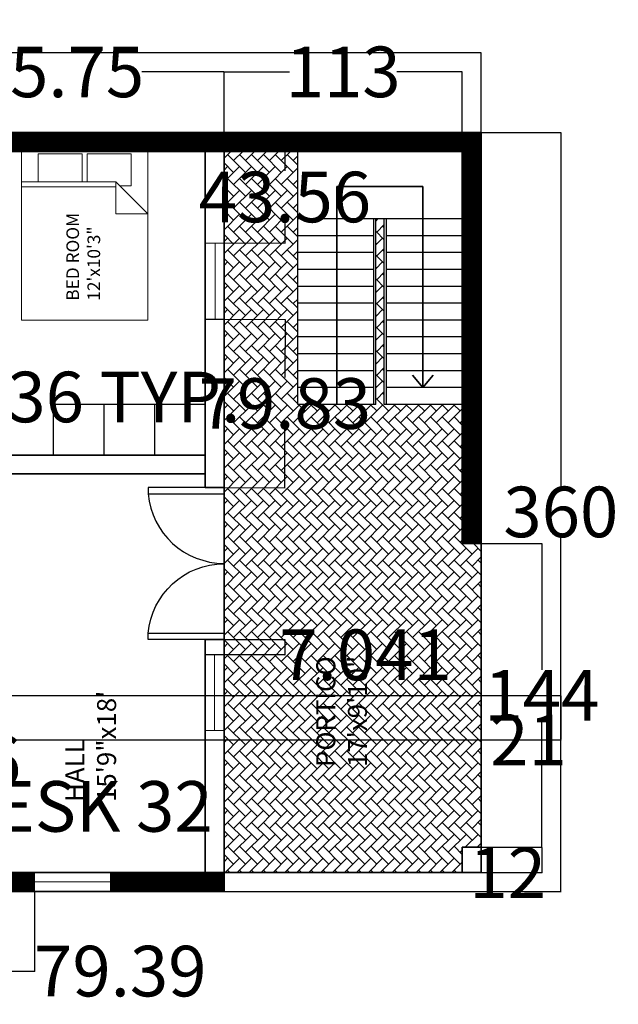
# Model space of a CAD drawing. Units: inches. Extents: x -1226 to 4538, y -998 to 1029.
# Tile 4 of 5: x -658 to -374, y -998 to -531. Entities that reach past the tile are written whole.
import ezdxf

# ---------------------------------------------------------------- set-up
doc = ezdxf.new("R2010")
doc.units = ezdxf.units.IN
doc.header["$MEASUREMENT"] = 0
for name, color, linetype, lineweight in [('A-ANNO-DIMS', 2, 'Continuous', 18), ('A-ANNO-SYMB', 7, 'Continuous', 35), ('A-AREA-IDEN', 7, 'Continuous', 18), ('A-DOOR', 4, 'Continuous', 25), ('A-FLOR-CASE', 8, 'Continuous', 25), ('A-FLOR-PATT', 2, 'Continuous', 13), ('A-FLOR-STRS', 7, 'Continuous', 25), ('A-FURN', 8, 'Continuous', 18), ('A-GLAZ', 3, 'Continuous', 18), ('A-WALL', 7, 'Continuous', 35), ('A-WALL-PATT', 1, 'Continuous', 13)]:
    doc.layers.add(name, color=color, linetype=linetype, lineweight=lineweight)
doc.styles.get("Standard").update_dxf_attribs({"font": 'arial.ttf'})
doc.dimstyles.get("Standard").update_dxf_attribs({"dimtxt": 24, "dimasz": 0.18, "dimexe": 0.18, "dimexo": 0.0625, "dimgap": 0.09, "dimtad": 0, "dimtih": 1, "dimtoh": 1, "dimdec": 0, "dimzin": 0, "dimdsep": 46, "dimlunit": 4, "dimtxsty": 'Standard', "dimcen": 0.09, "dimadec": 0, "dimazin": 0, "dimtfac": 1, "dimtdec": 0, "dimtofl": 0, "dimtmove": 0, "dimatfit": 3, "dimfxl": 1, "dimtolj": 1, "dimtzin": 0, "dimarcsym": 0})

# ---------------------------------------------------------------- blocks, each defined once
blk = doc.blocks.new('Bed - Queen')
for p, q in [((0, -80.00003), (0, 0)), ((0, 0), (59.99999, 0)), ((59.99999, 0), (59.99999, -80.00003)), ((7.99999, -1.2), (28.79998, -1.2)), ((7.99999, -14.4), (7.99999, -1.2)), ((28.79998, -1.2), (28.79998, -14.4)), ((31.19999, -1.2), (51.99999, -1.2)), ((31.19999, -14.4), (31.19999, -1.2)), ((51.99999, -1.2), (51.99999, -16.4)), ((0, -14.4), (44.8, -14.4)), ((44.8, -16.8), (0, -16.8)), ((59.99999, -29.6), (44.8, -14.4)), ((44.8, -14.4), (44.8, -29.6)), ((51.99999, -16.4), (46.79936, -16.4)), ((44.8, -29.6), (59.99999, -29.6)), ((59.99999, -80.00003), (0, -80.00003))]:
    blk.add_line(p, q)
blk = doc.blocks.new('DOOR-SWING-36')
for p, q in [((36, 36), (0, 36)), ((0, 36), (0, 33)), ((0, 33), (36, 33)), ((36, 33), (36, 36))]:
    blk.add_line(p, q)
blk.add_arc((36, 36.14), 36.14, 184.9791, 270)
blk = doc.blocks.new('WIN-36')
for p, q in [((0, 36), (9, 36)), ((4.5, 0), (4.5, 36)), ((0, 0), (9, 0))]:
    blk.add_line(p, q)
blk = doc.blocks.new('WARDROBE-72X24')
for p, q in [((72, 24), (0, 24)), ((0, 24), (0, 0)), ((24, 24), (24, 0)), ((48, 24), (48, 0)), ((72, 0), (72, 24)), ((0, 0), (72, 0))]:
    blk.add_line(p, q)
blk = doc.blocks.new('STAIR-RETURN-120X78')
for p, q in [((0, 0), (0, 120)), ((0, 120), (78, 120)), ((78, 120), (78, 0)), ((42, 88), (0, 88)), ((36, 0), (36, 88)), ((37, 0), (37, 88)), ((41, 0), (41, 88)), ((42, 0), (42, 88)), ((78, 88), (42, 88)), ((36, 80), (0, 80)), ((78, 80), (42, 80)), ((36, 72), (0, 72)), ((78, 72), (42, 72)), ((36, 64), (0, 64)), ((78, 64), (42, 64)), ((36, 56), (0, 56)), ((78, 56), (42, 56)), ((36, 48), (0, 48)), ((78, 48), (42, 48)), ((36, 40), (0, 40)), ((78, 40), (42, 40)), ((36, 32), (0, 32)), ((78, 32), (42, 32)), ((36, 24), (0, 24)), ((78, 24), (42, 24)), ((36, 16), (0, 16)), ((78, 16), (42, 16)), ((36, 8), (0, 8)), ((78, 8), (42, 8)), ((37, 0), (0, 0)), ((78, 0), (41, 0))]:
    blk.add_line(p, q)
blk = doc.blocks.new('STAIR-DIRECTION-RETURN')
for p, q in [((0, 0), (0, 103.3)), ((0, 103.3), (40.82, 103.3)), ((40.82, 103.3), (40.82, 8)), ((40.82, 8), (35.91, 13.94)), ((40.82, 8), (45.74, 13.94))]:
    blk.add_line(p, q)
blk = doc.blocks.new('*D26')
at = {"layer": 'A-ANNO-DIMS', "color": 0, "lineweight": -2, "transparency": 16777216}
for p, q in [((-694.2, -692), (-699.72, -692)), ((-699.54, -692.18), (-699.54, -697.48)), ((-699.54, -727.82), (-699.54, -722.51)), ((-694.2, -728), (-699.72, -728))]:
    blk.add_line(p, q, dxfattribs=at)
at = {"layer": 'A-ANNO-DIMS', "color": 0, "transparency": 16777216}
for points in [[(-699.57, -692.18), (-699.51, -692.18), (-699.54, -692)], [(-699.57, -727.82), (-699.51, -727.82), (-699.54, -728)]]:
    blk.add_solid(points, dxfattribs=at)
at = {"layer": 'Defpoints', "color": 0, "transparency": 16777216}
for p in [(-694.14, -692), (-699.54, -728), (-694.14, -728)]:
    blk.add_point(p, dxfattribs=at)
at = {"layer": 'A-ANNO-DIMS', "color": 0, "transparency": 16777216, "insert": (-699.54, -710), "char_height": 24, "attachment_point": 5}
blk.add_mtext('\\A1;DOOR LEAF 36 TYP.', dxfattribs=at)
blk = doc.blocks.new('*D44')
at = {"layer": 'A-ANNO-DIMS', "color": 0, "lineweight": -2, "transparency": 16777216}
for p, q in [((-728.59, -899.5), (-728.59, -904.39)), ((-696.71, -899.5), (-696.71, -904.39)), ((-728.41, -904.21), (-696.89, -904.21)), ((-696.71, -904.21), (-696.53, -904.21))]:
    blk.add_line(p, q, dxfattribs=at)
at = {"layer": 'A-ANNO-DIMS', "color": 0, "transparency": 16777216}
for points in [[(-728.41, -904.18), (-728.41, -904.24), (-728.59, -904.21)], [(-696.89, -904.18), (-696.89, -904.24), (-696.71, -904.21)]]:
    blk.add_solid(points, dxfattribs=at)
at = {"layer": 'Defpoints', "color": 0, "transparency": 16777216}
for p in [(-728.59, -899.43), (-696.71, -899.43), (-696.71, -904.21)]:
    blk.add_point(p, dxfattribs=at)
at = {"layer": 'A-ANNO-DIMS', "color": 0, "transparency": 16777216, "insert": (-629.67, -904.21), "char_height": 24, "attachment_point": 5}
blk.add_mtext('\\A1;DESK 32', dxfattribs=at)
blk = doc.blocks.new('*D45')
at = {"layer": 'A-ANNO-DIMS', "color": 0, "lineweight": -2, "transparency": 16777216}
for p, q in [((-696.65, -882.96), (-691.75, -882.96)), ((-691.93, -882.96), (-691.93, -882.78)), ((-691.93, -882.78), (-691.75, -882.78)), ((-691.93, -899.25), (-691.93, -883.14)), ((-696.65, -899.43), (-691.75, -899.43))]:
    blk.add_line(p, q, dxfattribs=at)
at = {"layer": 'A-ANNO-DIMS', "color": 0, "transparency": 16777216}
for points in [[(-691.96, -883.14), (-691.9, -883.14), (-691.93, -882.96)], [(-691.96, -899.25), (-691.9, -899.25), (-691.93, -899.43)]]:
    blk.add_solid(points, dxfattribs=at)
at = {"layer": 'Defpoints', "color": 0, "transparency": 16777216}
for p in [(-696.71, -882.96), (-691.93, -882.96), (-696.71, -899.43)]:
    blk.add_point(p, dxfattribs=at)
at = {"layer": 'A-ANNO-DIMS', "color": 0, "transparency": 16777216, "insert": (-675.61, -882.78), "char_height": 24, "attachment_point": 5}
blk.add_mtext('\\A1;16', dxfattribs=at)
blk = doc.blocks.new('*D48')
at = {"layer": 'A-ANNO-DIMS', "color": 0, "lineweight": -2, "transparency": 16777216}
for p, q in [((-1061.17, -584.46), (-1061.17, -546.6)), ((-1060.99, -546.78), (-776.71, -546.78)), ((-439.35, -546.78), (-723.62, -546.78)), ((-439.17, -584.46), (-439.17, -546.6))]:
    blk.add_line(p, q, dxfattribs=at)
at = {"layer": 'A-ANNO-DIMS', "color": 0, "transparency": 16777216}
for points in [[(-1060.99, -546.75), (-1060.99, -546.81), (-1061.17, -546.78)], [(-439.35, -546.75), (-439.35, -546.81), (-439.17, -546.78)]]:
    blk.add_solid(points, dxfattribs=at)
at = {"layer": 'Defpoints', "color": 0, "transparency": 16777216}
for p in [(-439.17, -546.78), (-1061.17, -584.53), (-439.17, -584.53)]:
    blk.add_point(p, dxfattribs=at)
at = {"layer": 'A-ANNO-DIMS', "color": 0, "transparency": 16777216, "insert": (-750.17, -546.78), "char_height": 24, "attachment_point": 5}
blk.add_mtext('\\A1;622', dxfattribs=at)
blk = doc.blocks.new('*D49')
at = {"layer": 'A-ANNO-DIMS', "color": 0, "lineweight": -2, "transparency": 16777216}
for p, q in [((-439.1, -584.53), (-401.24, -584.53)), ((-401.42, -584.71), (-401.42, -752.18)), ((-401.42, -944.35), (-401.42, -776.88)), ((-561.1, -944.53), (-401.24, -944.53))]:
    blk.add_line(p, q, dxfattribs=at)
at = {"layer": 'A-ANNO-DIMS', "color": 0, "transparency": 16777216}
for points in [[(-401.45, -584.71), (-401.39, -584.71), (-401.42, -584.53)], [(-401.45, -944.35), (-401.39, -944.35), (-401.42, -944.53)]]:
    blk.add_solid(points, dxfattribs=at)
at = {"layer": 'Defpoints', "color": 0, "transparency": 16777216}
for p in [(-439.17, -584.53), (-561.17, -944.53), (-401.42, -944.53)]:
    blk.add_point(p, dxfattribs=at)
at = {"layer": 'A-ANNO-DIMS', "color": 0, "transparency": 16777216, "insert": (-401.42, -764.53), "char_height": 24, "attachment_point": 5}
blk.add_mtext('\\A1;360', dxfattribs=at)
blk = doc.blocks.new('*D54')
at = {"layer": 'A-ANNO-DIMS', "color": 0, "lineweight": -2, "transparency": 16777216}
for p, q in [((-736.92, -593.48), (-736.92, -555.62)), ((-736.74, -555.8), (-697.91, -555.79)), ((-561.35, -555.78), (-600.18, -555.78)), ((-561.17, -593.46), (-561.17, -555.6))]:
    blk.add_line(p, q, dxfattribs=at)
at = {"layer": 'A-ANNO-DIMS', "color": 0, "transparency": 16777216}
for points in [[(-736.74, -555.77), (-736.74, -555.83), (-736.92, -555.8)], [(-561.35, -555.75), (-561.35, -555.81), (-561.17, -555.78)]]:
    blk.add_solid(points, dxfattribs=at)
at = {"layer": 'Defpoints', "color": 0, "transparency": 16777216}
for p in [(-561.17, -555.78), (-736.92, -593.55), (-561.17, -593.53)]:
    blk.add_point(p, dxfattribs=at)
at = {"layer": 'A-ANNO-DIMS', "color": 0, "transparency": 16777216, "insert": (-649.05, -555.79), "char_height": 24, "attachment_point": 5}
blk.add_mtext('\\A1;175.75', dxfattribs=at)
blk = doc.blocks.new('*D55')
at = {"layer": 'A-ANNO-DIMS', "color": 0, "lineweight": -2, "transparency": 16777216}
for p, q in [((-561.17, -593.46), (-561.17, -555.6)), ((-560.99, -555.78), (-530.14, -555.78)), ((-448.35, -555.78), (-479.19, -555.78)), ((-448.17, -593.46), (-448.17, -555.6))]:
    blk.add_line(p, q, dxfattribs=at)
at = {"layer": 'A-ANNO-DIMS', "color": 0, "transparency": 16777216}
for points in [[(-560.99, -555.75), (-560.99, -555.81), (-561.17, -555.78)], [(-448.35, -555.75), (-448.35, -555.81), (-448.17, -555.78)]]:
    blk.add_solid(points, dxfattribs=at)
at = {"layer": 'Defpoints', "color": 0, "transparency": 16777216}
for p in [(-448.17, -555.78), (-561.17, -593.53), (-448.17, -593.53)]:
    blk.add_point(p, dxfattribs=at)
at = {"layer": 'A-ANNO-DIMS', "color": 0, "transparency": 16777216, "insert": (-504.67, -555.78), "char_height": 24, "attachment_point": 5}
blk.add_mtext('\\A1;113', dxfattribs=at)
blk = doc.blocks.new('*D58')
at = {"layer": 'A-ANNO-DIMS', "color": 0, "lineweight": -2, "transparency": 16777216}
for p, q in [((-730.47, -944.64), (-730.47, -982.51)), ((-651.08, -944.55), (-651.08, -982.51)), ((-730.29, -982.33), (-651.26, -982.33)), ((-651.08, -982.33), (-650.9, -982.33))]:
    blk.add_line(p, q, dxfattribs=at)
at = {"layer": 'A-ANNO-DIMS', "color": 0, "transparency": 16777216}
for points in [[(-730.29, -982.3), (-730.29, -982.36), (-730.47, -982.33)], [(-651.26, -982.3), (-651.26, -982.36), (-651.08, -982.33)]]:
    blk.add_solid(points, dxfattribs=at)
at = {"layer": 'Defpoints', "color": 0, "transparency": 16777216}
for p in [(-730.47, -944.58), (-651.08, -944.48), (-651.08, -982.33)]:
    blk.add_point(p, dxfattribs=at)
at = {"layer": 'A-ANNO-DIMS', "color": 0, "transparency": 16777216, "insert": (-610.39, -982.33), "char_height": 24, "attachment_point": 5}
blk.add_mtext('\\A1;79.39', dxfattribs=at)
blk = doc.blocks.new('*D62')
at = {"layer": 'A-ANNO-DIMS', "color": 0, "lineweight": -2, "transparency": 16777216}
for p, q in [((-448.1, -779.53), (-410.24, -779.53)), ((-410.42, -779.71), (-410.42, -839.39)), ((-410.42, -923.35), (-410.42, -863.67)), ((-448.1, -923.53), (-410.24, -923.53))]:
    blk.add_line(p, q, dxfattribs=at)
at = {"layer": 'A-ANNO-DIMS', "color": 0, "transparency": 16777216}
for points in [[(-410.45, -779.71), (-410.39, -779.71), (-410.42, -779.53)], [(-410.45, -923.35), (-410.39, -923.35), (-410.42, -923.53)]]:
    blk.add_solid(points, dxfattribs=at)
at = {"layer": 'Defpoints', "color": 0, "transparency": 16777216}
for p in [(-448.17, -779.53), (-448.17, -923.53), (-410.42, -923.53)]:
    blk.add_point(p, dxfattribs=at)
at = {"layer": 'A-ANNO-DIMS', "color": 0, "transparency": 16777216, "insert": (-410.42, -851.53), "char_height": 24, "attachment_point": 5}
blk.add_mtext('\\A1;144', dxfattribs=at)
blk = doc.blocks.new('*D63')
at = {"layer": 'A-ANNO-DIMS', "color": 0, "lineweight": -2, "transparency": 16777216}
for p, q in [((-448.1, -923.53), (-410.24, -923.53)), ((-410.42, -923.71), (-410.42, -935.35)), ((-448.1, -935.53), (-410.24, -935.53)), ((-410.42, -935.71), (-410.6, -935.71)), ((-410.42, -935.53), (-410.42, -935.71))]:
    blk.add_line(p, q, dxfattribs=at)
at = {"layer": 'A-ANNO-DIMS', "color": 0, "transparency": 16777216}
for points in [[(-410.45, -923.71), (-410.39, -923.71), (-410.42, -923.53)], [(-410.45, -935.35), (-410.39, -935.35), (-410.42, -935.53)]]:
    blk.add_solid(points, dxfattribs=at)
at = {"layer": 'Defpoints', "color": 0, "transparency": 16777216}
for p in [(-448.17, -923.53), (-448.17, -935.53), (-410.42, -935.53)]:
    blk.add_point(p, dxfattribs=at)
at = {"layer": 'A-ANNO-DIMS', "color": 0, "transparency": 16777216, "insert": (-426.62, -935.71), "char_height": 24, "attachment_point": 5}
blk.add_mtext('\\A1;12', dxfattribs=at)
blk = doc.blocks.new('*D64')
at = {"layer": 'A-ANNO-DIMS', "color": 0, "lineweight": -2, "transparency": 16777216}
for p, q in [((-570.1, -593.53), (-532.24, -593.36)), ((-532.42, -593.54), (-532.37, -602.79)), ((-532.22, -636.74), (-532.26, -627.49)), ((-569.91, -637.09), (-532.04, -636.92))]:
    blk.add_line(p, q, dxfattribs=at)
at = {"layer": 'A-ANNO-DIMS', "color": 0, "transparency": 16777216}
for points in [[(-532.39, -593.54), (-532.45, -593.54), (-532.42, -593.36)], [(-532.19, -636.74), (-532.25, -636.74), (-532.22, -636.92)]]:
    blk.add_solid(points, dxfattribs=at)
at = {"layer": 'Defpoints', "color": 0, "transparency": 16777216}
for p in [(-570.17, -593.53), (-569.97, -637.09), (-532.22, -636.92)]:
    blk.add_point(p, dxfattribs=at)
at = {"layer": 'A-ANNO-DIMS', "color": 0, "transparency": 16777216, "insert": (-532.32, -615.14), "char_height": 24, "attachment_point": 5}
blk.add_mtext('\\A1;43.56', dxfattribs=at)
blk = doc.blocks.new('*D65')
at = {"layer": 'A-ANNO-DIMS', "color": 0, "lineweight": -2, "transparency": 16777216}
for p, q in [((-569.91, -673.09), (-532.04, -673.18)), ((-532.22, -673.36), (-532.29, -700.75)), ((-532.42, -752.84), (-532.35, -725.45)), ((-570.1, -752.93), (-532.24, -753.02))]:
    blk.add_line(p, q, dxfattribs=at)
at = {"layer": 'A-ANNO-DIMS', "color": 0, "transparency": 16777216}
for points in [[(-532.25, -673.36), (-532.19, -673.36), (-532.22, -673.18)], [(-532.45, -752.84), (-532.39, -752.84), (-532.42, -753.02)]]:
    blk.add_solid(points, dxfattribs=at)
at = {"layer": 'Defpoints', "color": 0, "transparency": 16777216}
for p in [(-569.97, -673.09), (-570.17, -752.93), (-532.42, -753.02)]:
    blk.add_point(p, dxfattribs=at)
at = {"layer": 'A-ANNO-DIMS', "color": 0, "transparency": 16777216, "insert": (-532.32, -713.1), "char_height": 24, "attachment_point": 5}
blk.add_mtext('\\A1;79.83', dxfattribs=at)
blk = doc.blocks.new('*D66')
at = {"layer": 'A-ANNO-DIMS', "color": 0, "lineweight": -2, "transparency": 16777216}
for p, q in [((-570.1, -825.1), (-532.24, -825.06)), ((-532.42, -825.24), (-532.41, -831.92)), ((-570.1, -832.14), (-532.23, -832.1)), ((-532.41, -832.1), (-532.41, -832.28)), ((-532.41, -832.28), (-532.23, -832.28))]:
    blk.add_line(p, q, dxfattribs=at)
at = {"layer": 'A-ANNO-DIMS', "color": 0, "transparency": 16777216}
for points in [[(-532.39, -825.24), (-532.45, -825.24), (-532.42, -825.06)], [(-532.38, -831.92), (-532.44, -831.92), (-532.41, -832.1)]]:
    blk.add_solid(points, dxfattribs=at)
at = {"layer": 'Defpoints', "color": 0, "transparency": 16777216}
for p in [(-570.17, -825.1), (-570.16, -832.14), (-532.41, -832.1)]:
    blk.add_point(p, dxfattribs=at)
at = {"layer": 'A-ANNO-DIMS', "color": 0, "transparency": 16777216, "insert": (-494.06, -832.28), "char_height": 24, "attachment_point": 5}
blk.add_mtext('\\A1;7.041', dxfattribs=at)
blk = doc.blocks.new('*D78')
at = {"layer": 'A-ANNO-DIMS', "color": 0, "lineweight": -2, "transparency": 16777216}
for p, q in [((-1028.09, -851.56), (-401.24, -851.56)), ((-401.42, -851.74), (-401.42, -872.38)), ((-1028.09, -872.56), (-401.24, -872.56)), ((-401.42, -872.74), (-401.6, -872.74)), ((-401.42, -872.56), (-401.42, -872.74))]:
    blk.add_line(p, q, dxfattribs=at)
at = {"layer": 'A-ANNO-DIMS', "color": 0, "transparency": 16777216}
for points in [[(-401.45, -851.74), (-401.39, -851.74), (-401.42, -851.56)], [(-401.45, -872.38), (-401.39, -872.38), (-401.42, -872.56)]]:
    blk.add_solid(points, dxfattribs=at)
at = {"layer": 'Defpoints', "color": 0, "transparency": 16777216}
for p in [(-1028.16, -851.56), (-1028.16, -872.56), (-401.42, -872.56)]:
    blk.add_point(p, dxfattribs=at)
at = {"layer": 'A-ANNO-DIMS', "color": 0, "transparency": 16777216, "insert": (-416.76, -872.74), "char_height": 24, "attachment_point": 5}
blk.add_mtext('\\A1;21', dxfattribs=at)

msp = doc.modelspace()

# ---------------------------------------------------------------- hatches: boundary and pattern name
at = {"layer": 'A-FLOR-PATT'}
h = msp.add_hatch(dxfattribs=at)
h.set_pattern_fill('AR-HBONE', color=256, angle=90)
h.set_pattern_definition([(135, (-1048.8063, 527.8678), (-5.656854, 3e-16), [12, -4]), (225, (-1051.6348, 530.696), (-5.656854, 8e-16), [12, -4])])
h.paths.add_polyline_path([(-526.1662, -713.5274), (-526.1662, -593.5274), (-561.1662, -593.5274), (-561.1662, -752.9256), (-561.1621, -752.9256), (-561.1621, -755.9256), (-561.1635, -822.1022), (-561.1621, -822.1022), (-561.1621, -825.1022), (-561.1658, -935.5274), (-448.1662, -935.5274), (-448.1662, -923.5274), (-439.1662, -923.5274), (-439.1662, -779.5274), (-448.1662, -779.5274), (-448.1662, -713.5274), (-485.1662, -713.5274), (-485.1662, -625.5274), (-489.1662, -625.5274), (-489.1662, -713.5274)])
h.paths.add_polyline_path([(-488.2978, -889.1778), (-488.2978, -827.0005), (-521.881, -827.0005), (-521.881, -889.1778)], flags=24)
at = {"layer": 'A-WALL-PATT'}
h = msp.add_hatch(dxfattribs=at)
h.set_pattern_fill('ANSI31', color=256, angle=90)
h.set_pattern_definition([(135, (-1048.80633, 527.86775), (-0.088388348, -0.088388348), [])])
h.paths.add_polyline_path([(-1052.1662, -935.5274), (-1052.1662, -878.4295), (-1061.1662, -878.4295), (-1061.1662, -944.5274), (-1012.2132, -944.5274), (-1012.2132, -935.5274)])
h.paths.add_polyline_path([(-976.2132, -935.5274), (-976.2132, -944.5274), (-730.4734, -944.5274), (-730.4734, -935.5274)])
h.paths.add_polyline_path([(-694.4734, -935.5274), (-694.4734, -944.5274), (-651.0832, -944.5274), (-651.0832, -935.5274)])
h.paths.add_polyline_path([(-615.0832, -935.5274), (-615.0832, -944.5274), (-561.1662, -944.5274), (-561.1662, -935.5274)])
h.paths.add_polyline_path([(-712.9165, -584.5274), (-712.9165, -593.5274), (-657.3138, -593.5274), (-657.3138, -593.4838), (-597.3139, -593.4838), (-448.1662, -593.5274), (-448.1662, -713.5274), (-448.1662, -779.5274), (-439.1662, -779.5274), (-439.1662, -584.5274)])
h.paths.add_polyline_path([(-875.9292, -584.5274), (-875.9292, -593.5274), (-736.9165, -593.5274), (-736.9165, -584.5274)])
h.paths.add_polyline_path([(-950.5052, -584.5274), (-950.5052, -593.5274), (-911.9292, -593.5274), (-911.9292, -584.5274)])
h.paths.add_polyline_path([(-1011.0429, -584.5274), (-1011.0429, -593.5274), (-974.5052, -593.5274), (-974.5052, -584.5274)])
h.paths.add_polyline_path([(-1061.1662, -584.5274), (-1061.1662, -693.4459), (-1052.1662, -693.4459), (-1052.1662, -593.5274), (-1035.0429, -593.5274), (-1035.0429, -584.5274)])
h.paths.add_polyline_path([(-1061.1662, -795.2404), (-1061.1662, -842.4295), (-1052.1662, -842.4295), (-1052.1662, -795.2404)])
h.paths.add_polyline_path([(-1061.1662, -717.4459), (-1061.1662, -739.4249), (-1052.1662, -739.4249), (-1052.1662, -717.4459)])

# ---------------------------------------------------------------- linework, layer by layer
at = {"layer": 'A-WALL'}
for p, q in [((-1061.1662, -584.5274), (-439.1662, -584.5274)), ((-439.1662, -935.5274), (-439.1662, -584.5274)), ((-1052.1662, -593.5274), (-448.1662, -593.5274)), ((-570.1662, -752.9256), (-570.1662, -593.5274)), ((-561.1662, -944.5274), (-561.1662, -593.5274)), ((-448.1662, -779.5274), (-448.1662, -593.5274)), ((-685.1662, -737.5274), (-570.1662, -737.5274)), ((-694.1662, -746.5274), (-570.1662, -746.5274)), ((-448.1662, -779.5274), (-439.1662, -779.5274)), ((-570.1662, -935.5274), (-570.1662, -825.1022)), ((-448.1662, -935.5274), (-448.1662, -923.5274)), ((-448.1662, -923.5274), (-439.1662, -923.5274)), ((-1052.1662, -935.5274), (-439.1662, -935.5274)), ((-1061.1662, -944.5274), (-561.1662, -944.5274))]:
    msp.add_line(p, q, dxfattribs=at)

# ---------------------------------------------------------------- block references
at = {"layer": 'A-ANNO-SYMB'}
msp.add_blockref('STAIR-DIRECTION-RETURN', (-507.666, -713.527), dxfattribs=at)
at = {"layer": 'A-DOOR'}
msp.add_blockref('DOOR-SWING-36', (-597.1617, -788.9258), dxfattribs=at)
at = {"layer": 'A-DOOR', "extrusion": (0, 0, -1), "zscale": -1, "rotation": 180}
msp.add_blockref('DOOR-SWING-36', (597.1617, -789.1021), dxfattribs=at)
at = {"layer": 'A-FLOR-CASE'}
msp.add_blockref('WARDROBE-72X24', (-642.1932, -737.5302), dxfattribs=at)
at = {"layer": 'A-FLOR-STRS'}
msp.add_blockref('STAIR-RETURN-120X78', (-526.166, -713.527), dxfattribs=at)
at = {"layer": 'A-FURN'}
msp.add_blockref('Bed - Queen', (-657.3138, -593.4838), dxfattribs=at)
at = {"layer": 'A-GLAZ'}
for p in [(-569.9717, -673.0906), (-570.1587, -868.1426)]:
    msp.add_blockref('WIN-36', p, dxfattribs=at)
at = {"layer": 'A-GLAZ', "rotation": 270.0000000000002}
msp.add_blockref('WIN-36', (-651.0827, -935.4839), dxfattribs=at)

# ---------------------------------------------------------------- texts
at = {"layer": 'A-AREA-IDEN', "attachment_point": 1, "rotation": 90}
for s, width, insert, char_height in [('BED ROOM\\P12\'x10\'3"', 53.566268, (-635.9672, -664.3267), 6), ('PORTICO\\P17\'x9\'10"', 76.603238, (-517.4086, -885.5588), 9), ('HALL\\P15\'9"x18\'', 76.603238, (-636.3964, -902.128), 9)]:
    msp.add_mtext_dynamic_manual_height_columns(s, width=width, gutter_width=1, heights=[0], dxfattribs=dict(at, insert=insert, char_height=char_height))

# ---------------------------------------------------------------- dimensions: what is measured, and where the dimension line sits
at = {"layer": 'A-ANNO-DIMS'}
for base, p1, p2, override, picture, middle in [((-439.1662, -546.7774), (-1061.1662, -584.5274), (-439.1662, -584.5274), {"dimdec": 0, "dimlfac": 1, "dimrnd": 0, "dimzin": 0, "dimdsep": 46, "dimlunit": 2}, '*D48', (-750.1662, -546.7774)), ((-448.1662, -555.7774), (-561.1662, -593.5274), (-448.1662, -593.5274), {"dimdec": 0, "dimlfac": 1, "dimrnd": 0, "dimzin": 0, "dimdsep": 46, "dimlunit": 2}, '*D55', (-504.6662, -555.7774)), ((-651.0832, -982.3314), (-730.4734, -944.5814), (-651.0832, -944.4838), {"dimdec": 2, "dimlfac": 1, "dimrnd": 0, "dimzin": 0, "dimdsep": 46, "dimlunit": 2}, '*D58', (-610.393, -982.3314))]:
    dim = msp.add_linear_dim(base=base, p1=p1, p2=p2, dimstyle='Standard', override=override, dxfattribs=at)
    dim.commit()
    dim.dimension.update_dxf_attribs({"geometry": picture, "text_midpoint": middle})
for base, p1, p2, angle, override, picture, middle in [((-561.1701, -555.7774), (-736.9165, -593.5456), (-561.1662, -593.5274), 0.005909, {"dimdec": 2, "dimlfac": 1, "dimrnd": 0, "dimzin": 0, "dimdsep": 46, "dimlunit": 2}, '*D54', (-649.0452, -555.7865)), ((-401.4162, -944.5274), (-439.1662, -584.5274), (-561.1662, -944.5274), 90, {"dimdec": 0, "dimlfac": 1, "dimrnd": 0, "dimzin": 0, "dimdsep": 46, "dimlunit": 2}, '*D49', (-401.4162, -764.5274)), ((-532.2221, -636.9226), (-570.1662, -593.5274), (-569.9718, -637.0911), 270.255669, {"dimdec": 2, "dimlfac": 1, "dimrnd": 0, "dimzin": 0, "dimdsep": 46, "dimlunit": 2}, '*D64', (-532.3193, -615.1408)), ((-532.4163, -753.0176), (-569.9718, -673.0911), (-570.1662, -752.9256), 269.860487, {"dimdec": 2, "dimlfac": 1, "dimrnd": 0, "dimzin": 0, "dimdsep": 46, "dimlunit": 2}, '*D65', (-532.3191, -713.1003)), ((-410.4162, -923.5274), (-448.1662, -779.5274), (-448.1662, -923.5274), 270, {"dimdec": 0, "dimlfac": 1, "dimrnd": 0, "dimzin": 0, "dimdsep": 46, "dimlunit": 2}, '*D62', (-410.4162, -851.5274)), ((-532.4087, -832.1031), (-570.1662, -825.1022), (-570.1587, -832.1431), 270.060667, {"dimdec": 3, "dimlfac": 1, "dimrnd": 0, "dimzin": 0, "dimdsep": 46, "dimlunit": 2}, '*D66', (-494.0594, -832.2831)), ((-401.4162, -872.5639), (-1028.1562, -851.5639), (-1028.1562, -872.5639), 90, {"dimdec": 0, "dimlfac": 1, "dimrnd": 0, "dimzin": 0, "dimdsep": 46, "dimlunit": 2}, '*D78', (-416.7639, -872.7439)), ((-691.9317, -882.9631), (-696.7132, -899.4326), (-696.7132, -882.9631), 90, {"dimdec": 0, "dimlfac": 1, "dimrnd": 0, "dimzin": 0, "dimdsep": 46, "dimlunit": 2}, '*D45', (-675.6099, -882.7831)), ((-410.4162, -935.5274), (-448.1662, -923.5274), (-448.1662, -935.5274), 270, {"dimdec": 0, "dimlfac": 1, "dimrnd": 0, "dimzin": 0, "dimdsep": 46, "dimlunit": 2}, '*D63', (-426.6234, -935.7074))]:
    dim = msp.add_linear_dim(base=base, p1=p1, p2=p2, angle=angle, dimstyle='Standard', override=override, dxfattribs=at)
    dim.commit()
    dim.dimension.update_dxf_attribs({"geometry": picture, "text_midpoint": middle})
dim = msp.add_linear_dim(base=(-699.5403, -727.9957), p1=(-694.1403, -691.9957), p2=(-694.1403, -727.9957), angle=270, text='DOOR LEAF <> TYP.', dimstyle='Standard', override={"dimdec": 0, "dimlfac": 1, "dimrnd": 0, "dimzin": 0, "dimdsep": 46, "dimlunit": 2}, dxfattribs=at)
dim.commit()
dim.dimension.update_dxf_attribs({"geometry": '*D26', "text_midpoint": (-699.5403, -709.9957)})
dim = msp.add_linear_dim(base=(-696.7132, -904.2141), p1=(-728.5897, -899.4326), p2=(-696.7132, -899.4326), text='DESK <>', dimstyle='Standard', override={"dimdec": 0, "dimlfac": 1, "dimrnd": 0, "dimzin": 0, "dimdsep": 46, "dimlunit": 2}, dxfattribs=at)
dim.commit()
dim.dimension.update_dxf_attribs({"geometry": '*D44', "text_midpoint": (-629.6656, -904.2141)})

doc.saveas('drawing.dxf')
